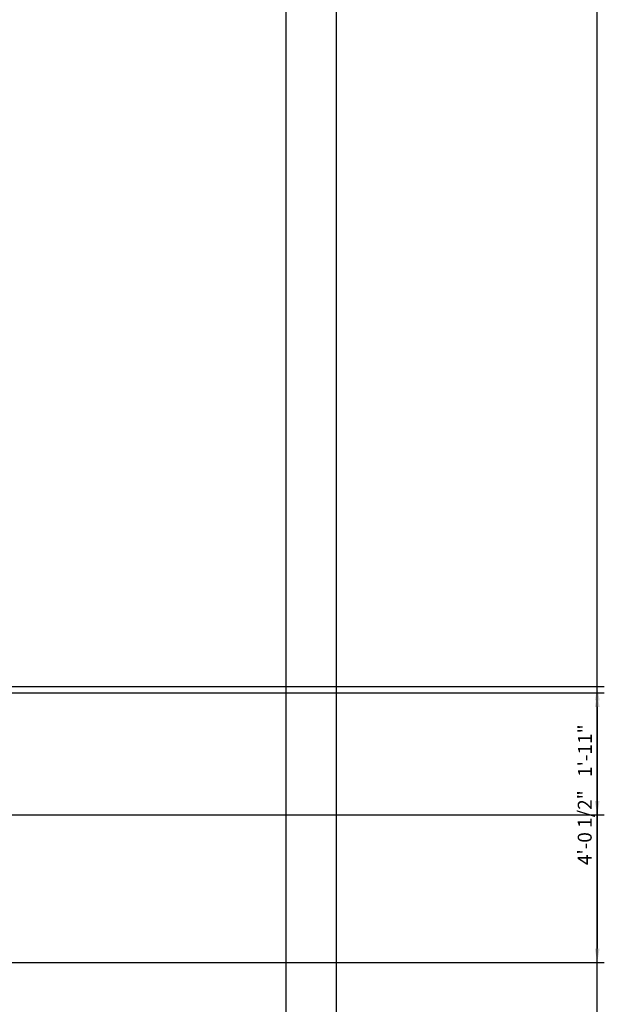
# Model space of a CAD drawing. Units: inches. Extents: x 1624 to 3956, y 1589 to 5028.
# Tile 15 of 16: x 2113 to 2218, y 2250 to 2426. Entities that reach past the tile are written whole.
import ezdxf

# ---------------------------------------------------------------- set-up
doc = ezdxf.new("R2010")
doc.units = ezdxf.units.IN
doc.layers.add('A-ANNO-DIMS', color=2, linetype='Continuous', lineweight=13)
doc.layers.add('C-PROP', color=7, linetype='Continuous', lineweight=25)
doc.styles.get("Standard").update_dxf_attribs({"font": 'arial.ttf'})
doc.dimstyles.new('Copy of ISO-25', dxfattribs={"dimtxt": 2.5, "dimasz": 2.5, "dimexe": 1.25, "dimexo": 0.625, "dimtad": 1, "dimdec": 1, "dimlunit": 4, "dimtxsty": 'Standard', "dimcen": 2.5, "dimadec": 0, "dimazin": 0, "dimtfac": 1, "dimtdec": 1, "dimtmove": 0, "dimatfit": 3, "dimfxl": 1, "dimarcsym": 0})

# ---------------------------------------------------------------- blocks, each defined once
blk = doc.blocks.new('*D67')
at = {"layer": 'A-ANNO-DIMS', "color": 0, "lineweight": -2, "transparency": 16777216}
for p, q in [((2170.2, 2564.79), (2217.63, 2564.79)), ((2216.38, 1649.29), (2216.38, 2562.29)), ((2170.2, 1646.79), (2217.63, 1646.79))]:
    blk.add_line(p, q, dxfattribs=at)
at = {"layer": 'A-ANNO-DIMS', "color": 0, "transparency": 16777216}
for points in [[(2215.96, 2562.29), (2216.8, 2562.29), (2216.38, 2564.79)], [(2215.96, 1649.29), (2216.8, 1649.29), (2216.38, 1646.79)]]:
    blk.add_solid(points, dxfattribs=at)
at = {"layer": 'Defpoints', "color": 0, "transparency": 16777216}
for p in [(2169.58, 2564.79), (2216.38, 2564.79), (2169.58, 1646.79)]:
    blk.add_point(p, dxfattribs=at)
at = {"layer": 'A-ANNO-DIMS', "color": 0, "transparency": 16777216, "insert": (2214.48, 2105.79), "char_height": 2.5, "attachment_point": 5, "rotation": 90}
blk.add_mtext('76\'-6"', dxfattribs=at)
blk = doc.blocks.new('*D96')
at = {"layer": 'A-ANNO-DIMS', "color": 0, "lineweight": -2, "transparency": 16777216}
for p, q in [((1952.2, 2305.65), (2217.63, 2305.65)), ((2216.38, 2303.15), (2216.38, 2259.79)), ((1998.67, 2257.29), (2217.63, 2257.29))]:
    blk.add_line(p, q, dxfattribs=at)
at = {"layer": 'A-ANNO-DIMS', "color": 0, "transparency": 16777216}
for points in [[(2215.96, 2303.15), (2216.8, 2303.15), (2216.38, 2305.65)], [(2215.96, 2259.79), (2216.8, 2259.79), (2216.38, 2257.29)]]:
    blk.add_solid(points, dxfattribs=at)
at = {"layer": 'Defpoints', "color": 0, "transparency": 16777216}
for p in [(1951.58, 2305.65), (1998.04, 2257.29), (2216.38, 2257.29)]:
    blk.add_point(p, dxfattribs=at)
at = {"layer": 'A-ANNO-DIMS', "color": 0, "transparency": 16777216, "insert": (2214.46, 2281.47), "char_height": 2.5, "attachment_point": 5, "rotation": 90}
blk.add_mtext('4\'-0 1/2"', dxfattribs=at)
blk = doc.blocks.new('*D100')
at = {"layer": 'A-ANNO-DIMS', "color": 0, "lineweight": -2, "transparency": 16777216}
for p, q in [((1738.2, 2306.79), (2217.63, 2306.79)), ((2216.38, 2286.28), (2216.38, 2304.29)), ((1761.2, 2283.78), (2217.63, 2283.78))]:
    blk.add_line(p, q, dxfattribs=at)
at = {"layer": 'A-ANNO-DIMS', "color": 0, "transparency": 16777216}
for points in [[(2215.96, 2304.29), (2216.8, 2304.29), (2216.38, 2306.79)], [(2215.96, 2286.28), (2216.8, 2286.28), (2216.38, 2283.78)]]:
    blk.add_solid(points, dxfattribs=at)
at = {"layer": 'Defpoints', "color": 0, "transparency": 16777216}
for p in [(1737.58, 2306.79), (2216.38, 2306.79), (1760.58, 2283.78)]:
    blk.add_point(p, dxfattribs=at)
at = {"layer": 'A-ANNO-DIMS', "color": 0, "transparency": 16777216, "insert": (2214.5, 2295.29), "char_height": 2.5, "attachment_point": 5, "rotation": 90}
blk.add_mtext('1\'-11"', dxfattribs=at)

msp = doc.modelspace()

# ---------------------------------------------------------------- linework, layer by layer
at = {"layer": 'C-PROP'}
for p, q in [((2169.58, 1652.79), (2169.58, 2559.46)), ((2160.58, 1652.79), (2160.58, 2555.79))]:
    msp.add_line(p, q, dxfattribs=at)

# ---------------------------------------------------------------- dimensions: what is measured, and where the dimension line sits
at = {"layer": 'A-ANNO-DIMS'}
for base, p1, p2, picture, middle in [((2216.38, 2564.79), (2169.58, 1646.79), (2169.58, 2564.79), '*D67', (2214.48, 2105.79)), ((2216.38, 2306.79), (1760.58, 2283.78), (1737.58, 2306.79), '*D100', (2214.5, 2295.29)), ((2216.38, 2257.29), (1951.58, 2305.65), (1998.04, 2257.29), '*D96', (2214.46, 2281.47))]:
    dim = msp.add_linear_dim(base=base, p1=p1, p2=p2, angle=90, dimstyle='Copy of ISO-25', override={"dimdec": 1, "dimlfac": 1, "dimrnd": 0, "dimzin": 1, "dimdsep": 46, "dimlunit": 4, "dimfrac": 2}, dxfattribs=at)
    dim.commit()
    dim.dimension.update_dxf_attribs({"geometry": picture, "text_midpoint": middle})

doc.saveas('drawing.dxf')
